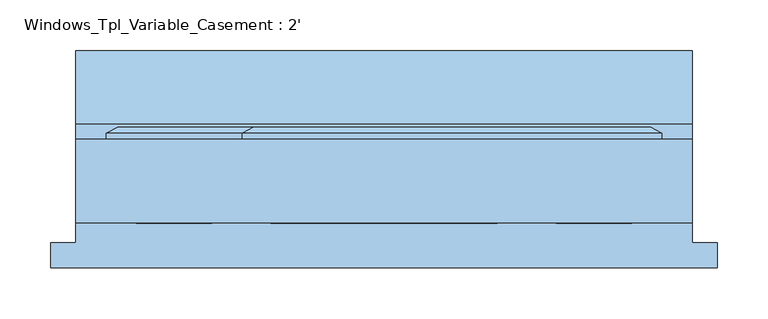
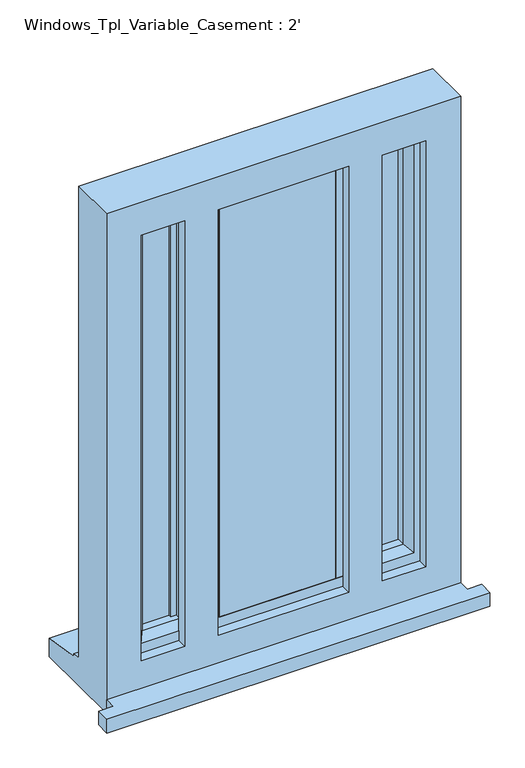
"""IFC4 building model written with IfcOpenShell, lengths in millimetres: window geometry, Windows_Tpl_Variable_Casement : 2'."""

from ifc_helpers import new_model, si_unit, frame, origin, place, context, project, spatial, polyline, outline, extrude, faceted_brep, source, transform, mapped, element, save


def windows_tpl_variable_casement_2_47b04551(model_context):
    return source(origin(), model_context, "Body", "SolidModel", [
        extrude(outline(polyline([(-319.6, -92.7434322), (-319.6, -67.7434322), (-294.6, -67.7434322), (-294.6, -48.3434322), (315.0, -48.3434322), (315.0, -67.7434322), (340.0, -67.7434322), (340.0, -92.7434322), (-319.6, -92.7434322)])), frame((0.0, 0.0, 1200.0), z_axis=(0.0, 0.0, 1.0), x_axis=(1.0, 0.0, 0.0)), (0.0, 0.0, 1.0), 25.0),
        faceted_brep([(-130.0, 34.6565678, 2080.0), (-130.0, 40.4300705, 2080.0), (-130.0, 40.4300705, 1253.0), (-130.0, 34.6565678, 1253.0), (-120.0, -30.3434322, 2070.0), (-120.0, 34.6565678, 2070.0), (-120.0, 34.6565678, 1263.0), (-120.0, -30.3434322, 1263.0), (-80.0, -15.8505323, 2030.0), (-90.1480377, -30.3434322, 2040.1480377), (-90.1480377, -30.3434322, 1292.8519623), (-80.0, -15.8505323, 1303.0), (-80.0, -1.3434322, 2030.0), (-80.0, -1.3434322, 1303.0), (-90.0, 22.6565678, 2040.0), (-90.0, -1.3434322, 2040.0), (-90.0, -1.3434322, 1293.0), (-90.0, 22.6565678, 1293.0), (-80.0, 40.4300705, 2030.0), (-80.0, 22.6565678, 2030.0), (-80.0, 22.6565678, 1303.0), (-80.0, 40.4300705, 1303.0), (-97.4457548, 46.2035732, 2047.4457548), (-97.4457548, 46.2035732, 1285.5542452), (-119.2153903, 46.2035732, 2069.2153903), (-119.2153903, 46.2035732, 1263.7846097), (285.0, 40.4300705, 1253.0), (285.0, 34.6565678, 1253.0), (275.0, 34.6565678, 1263.0), (275.0, -30.3434322, 1263.0), (245.1480377, -30.3434322, 1292.8519623), (235.0, -15.8505323, 1303.0), (235.0, -1.3434322, 1303.0), (245.0, -1.3434322, 1293.0), (245.0, 22.6565678, 1293.0), (235.0, 22.6565678, 1303.0), (235.0, 40.4300705, 1303.0), (252.4457548, 46.2035732, 1285.5542452), (274.2153903, 46.2035732, 1263.7846097), (285.0, 40.4300705, 2080.0), (285.0, 34.6565678, 2080.0), (275.0, 34.6565678, 2070.0), (275.0, -30.3434322, 2070.0), (245.1480377, -30.3434322, 2040.1480377), (235.0, -15.8505323, 2030.0), (235.0, -1.3434322, 2030.0), (245.0, -1.3434322, 2040.0), (245.0, 22.6565678, 2040.0), (235.0, 22.6565678, 2030.0), (235.0, 40.4300705, 2030.0), (252.4457548, 46.2035732, 2047.4457548), (274.2153903, 46.2035732, 2069.2153903)], [[[0, 1, 2, 3]], [[4, 5, 6, 7]], [[8, 9, 10, 11]], [[12, 8, 11, 13]], [[14, 15, 16, 17]], [[18, 19, 20, 21]], [[22, 18, 21, 23]], [[1, 24, 25, 2]], [[3, 2, 26, 27]], [[7, 6, 28, 29]], [[11, 10, 30, 31]], [[13, 11, 31, 32]], [[17, 16, 33, 34]], [[21, 20, 35, 36]], [[23, 21, 36, 37]], [[2, 25, 38, 26]], [[27, 26, 39, 40]], [[29, 28, 41, 42]], [[31, 30, 43, 44]], [[32, 31, 44, 45]], [[34, 33, 46, 47]], [[36, 35, 48, 49]], [[37, 36, 49, 50]], [[26, 38, 51, 39]], [[40, 39, 1, 0]], [[3, 27, 40, 0], [5, 41, 28, 6]], [[42, 41, 5, 4]], [[7, 29, 42, 4], [9, 43, 30, 10]], [[44, 43, 9, 8]], [[45, 44, 8, 12]], [[15, 46, 33, 16], [13, 32, 45, 12]], [[47, 46, 15, 14]], [[17, 34, 47, 14], [19, 48, 35, 20]], [[49, 48, 19, 18]], [[50, 49, 18, 22]], [[24, 51, 38, 25], [23, 37, 50, 22]], [[39, 51, 24, 1]]]),
        faceted_brep([(150.4, 34.6565678, 2080.0), (150.4, 40.4300705, 2080.0), (-264.6, 40.4300705, 2080.0), (-264.6, 34.6565678, 2080.0), (140.4, -30.3434322, 2070.0), (140.4, 34.6565678, 2070.0), (-254.6, 34.6565678, 2070.0), (-254.6, -30.3434322, 2070.0), (100.4, -15.8505323, 2030.0), (110.5480377, -30.3434322, 2040.1480377), (-224.7480377, -30.3434322, 2040.1480377), (-214.6, -15.8505323, 2030.0), (100.4, -1.3434322, 2030.0), (-214.6, -1.3434322, 2030.0), (110.4, 22.6565678, 2040.0), (110.4, -1.3434322, 2040.0), (-224.6, -1.3434322, 2040.0), (-224.6, 22.6565678, 2040.0), (100.4, 40.4300705, 2030.0), (100.4, 22.6565678, 2030.0), (-214.6, 22.6565678, 2030.0), (-214.6, 40.4300705, 2030.0), (119.2145656, 46.2035732, 2048.8145656), (-233.4145656, 46.2035732, 2048.8145656), (138.7692194, 46.2035732, 2068.3692194), (-252.9692194, 46.2035732, 2068.3692194), (-264.6, 40.4300705, 1253.0), (-264.6, 34.6565678, 1253.0), (-254.6, 34.6565678, 1263.0), (-254.6, -30.3434322, 1263.0), (-224.7480377, -30.3434322, 1292.8519623), (-214.6, -15.8505323, 1303.0), (-214.6, -1.3434322, 1303.0), (-224.6, -1.3434322, 1293.0), (-224.6, 22.6565678, 1293.0), (-214.6, 22.6565678, 1303.0), (-214.6, 40.4300705, 1303.0), (-233.4145656, 46.2035732, 1284.1854344), (-252.9692194, 46.2035732, 1264.6307806), (150.4, 40.4300705, 1253.0), (150.4, 34.6565678, 1253.0), (140.4, 34.6565678, 1263.0), (140.4, -30.3434322, 1263.0), (110.5480377, -30.3434322, 1292.8519623), (100.4, -15.8505323, 1303.0), (100.4, -1.3434322, 1303.0), (110.4, -1.3434322, 1293.0), (110.4, 22.6565678, 1293.0), (100.4, 22.6565678, 1303.0), (100.4, 40.4300705, 1303.0), (119.2145656, 46.2035732, 1284.1854344), (138.7692194, 46.2035732, 1264.6307806)], [[[0, 1, 2, 3]], [[4, 5, 6, 7]], [[8, 9, 10, 11]], [[12, 8, 11, 13]], [[14, 15, 16, 17]], [[18, 19, 20, 21]], [[22, 18, 21, 23]], [[1, 24, 25, 2]], [[3, 2, 26, 27]], [[7, 6, 28, 29]], [[11, 10, 30, 31]], [[13, 11, 31, 32]], [[17, 16, 33, 34]], [[21, 20, 35, 36]], [[23, 21, 36, 37]], [[2, 25, 38, 26]], [[27, 26, 39, 40]], [[0, 3, 27, 40], [41, 28, 6, 5]], [[29, 28, 41, 42]], [[4, 7, 29, 42], [43, 30, 10, 9]], [[31, 30, 43, 44]], [[32, 31, 44, 45]], [[46, 33, 16, 15], [12, 13, 32, 45]], [[34, 33, 46, 47]], [[14, 17, 34, 47], [48, 35, 20, 19]], [[36, 35, 48, 49]], [[37, 36, 49, 50]], [[51, 38, 25, 24], [22, 23, 37, 50]], [[26, 38, 51, 39]], [[40, 39, 1, 0]], [[42, 41, 5, 4]], [[44, 43, 9, 8]], [[45, 44, 8, 12]], [[47, 46, 15, 14]], [[49, 48, 19, 18]], [[50, 49, 18, 22]], [[39, 51, 24, 1]]]),
        faceted_brep([(315.0, -48.3434322, 2110.0), (-294.6, -48.3434322, 2110.0), (-294.6, -48.3434322, 1200.0), (315.0, -48.3434322, 1200.0), (255.0, -48.3434322, 2050.0), (255.0, -48.3434322, 1275.0), (180.4, -48.3434322, 1275.0), (180.4, -48.3434322, 2050.0), (-160.0, -48.3434322, 2050.0), (-160.0, -48.3434322, 1275.0), (-234.6, -48.3434322, 1275.0), (-234.6, -48.3434322, 2050.0), (122.4, -48.3434322, 2050.0), (122.4, -48.3434322, 1275.0), (-102.0, -48.3434322, 1275.0), (-102.0, -48.3434322, 2050.0), (-294.6, 34.6565678, 2110.0), (-294.6, 34.6565678, 1251.0), (-294.6, 49.6565678, 1249.68767), (-294.6, 49.6565678, 1244.7449676), (-294.6, 122.1565678, 1233.8088847), (-294.6, 122.1565678, 1200.0), (315.0, 34.6565678, 2110.0), (315.0, 34.6565678, 1251.0), (-254.6, 34.6565678, 2070.0), (-254.6, 34.6565678, 1263.0), (-160.0, 34.6565678, 1263.0), (-160.0, 34.6565678, 2070.0), (180.4, 34.6565678, 2070.0), (180.4, 34.6565678, 1263.0), (275.0, 34.6565678, 1263.0), (275.0, 34.6565678, 2070.0), (-120.0, 34.6565678, 2070.0), (-120.0, 34.6565678, 1263.0), (140.4, 34.6565678, 1263.0), (140.4, 34.6565678, 2070.0), (-254.6, -30.3434322, 2070.0), (-254.6, -30.3434322, 1263.0), (-150.0, -30.3434322, 2070.0), (-150.0, -30.3434322, 1263.0), (-160.0, -30.3434322, 2050.0), (-234.6, -30.3434322, 2050.0), (-234.6, -30.3434322, 1275.0), (-160.0, -30.3434322, 1275.0), (-120.0, -30.3434322, 2070.0), (140.4, -30.3434322, 2070.0), (140.4, -30.3434322, 1263.0), (-120.0, -30.3434322, 1263.0), (122.4, -30.3434322, 2050.0), (-102.0, -30.3434322, 2050.0), (-102.0, -30.3434322, 1275.0), (122.4, -30.3434322, 1275.0), (170.4, -30.3434322, 2070.0), (275.0, -30.3434322, 2070.0), (275.0, -30.3434322, 1263.0), (170.4, -30.3434322, 1263.0), (255.0, -30.3434322, 2050.0), (180.4, -30.3434322, 2050.0), (180.4, -30.3434322, 1275.0), (255.0, -30.3434322, 1275.0), (-160.0, -6.3434322, 2070.0), (-150.0, -6.3434322, 2070.0), (170.4, -6.3434322, 2070.0), (180.4, -6.3434322, 2070.0), (315.0, 122.1565678, 1200.0), (315.0, 122.1565678, 1233.8088847), (315.0, 49.6565678, 1244.7449676), (315.0, 49.6565678, 1249.68767), (180.4, -6.3434322, 1263.0), (170.4, -6.3434322, 1263.0), (-150.0, -6.3434322, 1263.0), (-160.0, -6.3434322, 1263.0)], [[[0, 1, 2, 3], [4, 5, 6, 7], [8, 9, 10, 11], [12, 13, 14, 15]], [[2, 1, 16, 17, 18, 19, 20, 21]], [[17, 16, 22, 23], [24, 25, 26, 27], [28, 29, 30, 31], [32, 33, 34, 35]], [[25, 24, 36, 37]], [[36, 38, 39, 37], [40, 41, 42, 43]], [[44, 45, 46, 47], [48, 49, 50, 51]], [[52, 53, 54, 55], [56, 57, 58, 59]], [[41, 11, 10, 42]], [[1, 0, 22, 16]], [[36, 24, 27, 60, 61, 38]], [[35, 45, 44, 32]], [[31, 53, 52, 62, 63, 28]], [[11, 41, 40, 8]], [[48, 12, 15, 49]], [[56, 4, 7, 57]], [[23, 22, 0, 3, 64, 65, 66, 67]], [[31, 30, 54, 53]], [[4, 56, 59, 5]], [[57, 7, 6, 58]], [[12, 48, 51, 13]], [[35, 34, 46, 45]], [[29, 28, 63, 68]], [[68, 63, 62, 69]], [[69, 62, 52, 55]], [[61, 70, 39, 38]], [[70, 61, 60, 71]], [[71, 60, 27, 26]], [[33, 32, 44, 47]], [[49, 15, 14, 50]], [[8, 40, 43, 9]], [[64, 3, 2, 21]], [[65, 64, 21, 20]], [[66, 65, 20, 19]], [[67, 66, 19, 18]], [[23, 67, 18, 17]], [[26, 25, 37, 39, 70, 71]], [[34, 33, 47, 46]], [[55, 54, 30, 29, 68, 69]], [[6, 5, 59, 58]], [[14, 13, 51, 50]], [[43, 42, 10, 9]]]),
        extrude(outline(polyline([(110.4, -1.3434322), (-224.6, -1.3434322), (-224.6, 22.6565678), (110.4, 22.6565678), (110.4, -1.3434322)])), frame((0.0, 0.0, 1293.0), z_axis=(0.0, 0.0, 1.0), x_axis=(1.0, 0.0, 0.0)), (0.0, 0.0, 1.0), 747.0),
        extrude(outline(polyline([(-150.0, -6.3434322), (170.4, -6.3434322), (170.4, -30.3434322), (-150.0, -30.3434322), (-150.0, -6.3434322)])), frame((0.0, 0.0, 1263.0), z_axis=(0.0, 0.0, 1.0), x_axis=(1.0, 0.0, 0.0)), (0.0, 0.0, 1.0), 807.0),
        extrude(outline(polyline([(245.0, -1.3434322), (-90.0, -1.3434322), (-90.0, 22.6565678), (245.0, 22.6565678), (245.0, -1.3434322)])), frame((0.0, 0.0, 1293.0), z_axis=(0.0, 0.0, 1.0), x_axis=(1.0, 0.0, 0.0)), (0.0, 0.0, 1.0), 747.0),
    ])


if __name__ == "__main__":
    model = new_model("IFC4")
    model_context = context("Model", 3, world=origin())
    ifc_project = project(units=[si_unit("LENGTHUNIT", "METRE", prefix="MILLI")], contexts=[model_context])
    site = spatial("IfcSite", under=ifc_project)
    building = spatial("IfcBuilding", under=site)
    placement = place(None, origin())
    windows_tpl_variable_casement_2_shape = windows_tpl_variable_casement_2_47b04551(model_context)
    element("IfcWindow", 1, ObjectType="Windows_Tpl_Variable_Casement : 2'", at=placement, inside=building, context=model_context, shape_type="MappedRepresentation", body=[
        mapped(windows_tpl_variable_casement_2_shape, transform((0.0, 0.0, 0.0), x_axis=(1.0, 0.0, 0.0), y_axis=(0.0, 1.0, 0.0), z_axis=(0.0, 0.0, 1.0))),
    ])
    save(model, "model.ifc")

# Revit data of these elements
# Type "Windows_Tpl_Variable_Casement : 2'"
#   Type Mark = "82"
#   Operation = "TriplePanelVertical"
#   Construction Type Id = "GSP4R"
#   Manufacturer = "Revit"
#   Keynote = "L10"
#   Analytic Construction = "1/8 in Pilkington single glazing"
#   Wrap Layers (Int) from Ext = 177.5 mm
#   Wrap Layers (Ext) from Ext = 102.5 mm
#   Window Board Projection = 25 mm
#   Window Board Extension = 25 mm
#   Visual Light Transmittance = 0.9
#   Solar Heat Gain Coefficient = 0.78
#   Rough Width = 609.6 mm
#   Rough Height = 910 mm
#   Height = 910 mm
#   Width = 609.6 mm
#   Heat Transfer Coefficient (U) = 3.6886 W/(m²·K)
#   Glazing Thickness = 24 mm
#   FrameOffset - External = 50 mm
#   Frame Depth = 65 mm
#   Default Head Height = 2110 mm
#   Cill Depth = 87.5 mm
#   Cavity Closer Width = 50 mm
#   Cavity Closer Offset from Ext = 102.5 mm
#   Cavity Closer Depth = 85 mm
#   Casement Width = 450 mm
#   Vis - Cavity Closers = yes
#   Define Thermal Properties by = 1
#   Material Trim = Window Frame
#   Material Glass = Glass
#   Material Frame = Window Frame
#   Wall Closure = (empty or 0)
# Element 1 (IfcWindow, "Windows_Tpl_Variable_Casement : 2'")
#   Materials on its faces: "Window Frame", "Glass"
# Materials
#   "Window Frame": colour RGB 249 249 249, transparency 0, Keynote = "L10", Cost = 0
#   "Glass": class "Glass", colour RGB 0 128 192, transparency 0.9, Description = "Soda Lime Glass", Cost = 0
